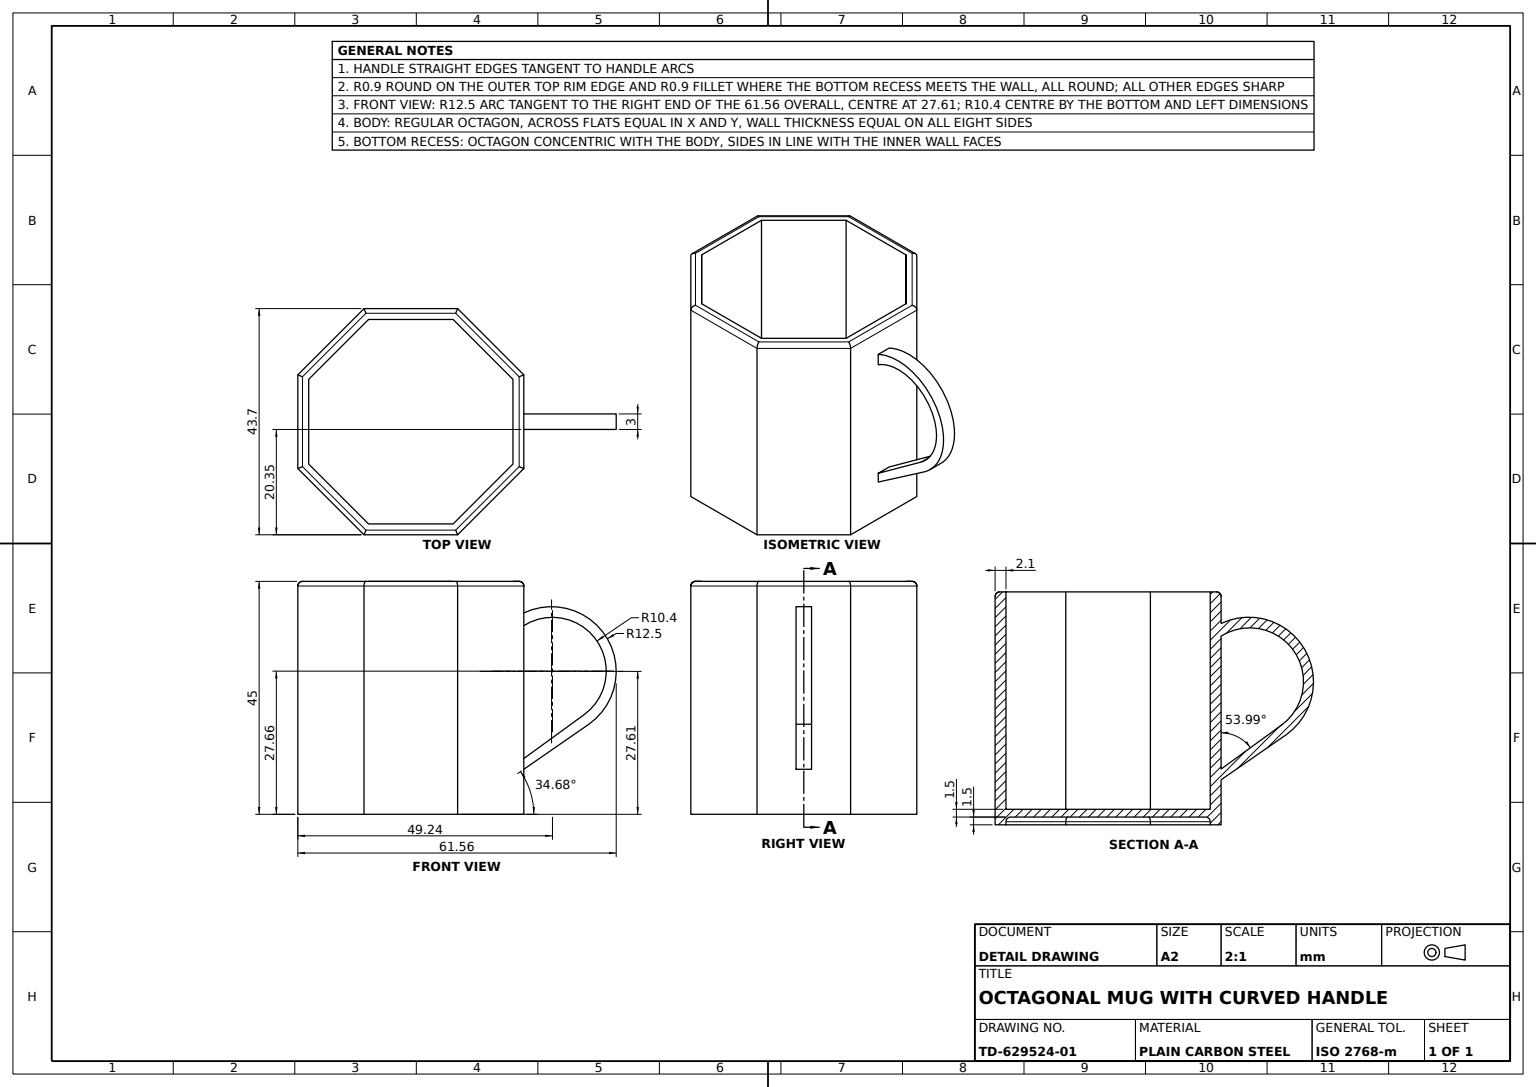
from build123d import *

# Parameters (mm, degrees)
OCTAGON_WALL_45MM_DEPTH    = 45
BOTTOM_START               = -3
BOTTOM_PLATE_1_5MM_DEPTH   = 1.5
BOTTOM_PLATE_FILLET_R0_9_R = 0.9
HANDLE_3MM_DEPTH           = 1.5
WALL_EDGE_FILLET_R0_9_R    = 0.9


with BuildPart() as part:
    # Octagon Wall Profile → Octagon Wall 45mm (new body)
    with BuildSketch(Plane(origin=(0, 0, 0), x_dir=(1, 0, 0), z_dir=(0, 1, 0))):
        Polygon((21.848632739, -9.05), (21.848632739, 9.05), (9.05, 21.848632739), (-9.05, 21.848632739), (-21.848632739, 9.05), (-21.848632739, -9.05), (-9.05, -21.848632739), (9.05, -21.848632739), align=None)
        Polygon((-19.748632739, 8.180151519), (-19.748632739, -8.180151519), (-8.180151519, -19.748632739), (8.180151519, -19.748632739), (19.748632739, -8.180151519), (19.748632739, 8.180151519), (8.180151519, 19.748632739), (-8.180151519, 19.748632739), align=None, mode=Mode.SUBTRACT)
    extrude(amount=OCTAGON_WALL_45MM_DEPTH)

    # Bottom Plate Profile → Bottom Plate 1.5mm (add)
    with BuildSketch(Plane.XZ.offset(BOTTOM_START)):
        Polygon((19.748632739, -8.180151519), (19.748632739, 8.180151519), (8.180151519, 19.748632739), (-8.180151519, 19.748632739), (-19.748632739, 8.180151519), (-19.748632739, -8.180151519), (-8.180151519, -19.748632739), (8.180151519, -19.748632739), align=None)
    extrude(amount=BOTTOM_PLATE_1_5MM_DEPTH)

    # Bottom Plate Fillet R0.9
    bottom_plate_fillet_r0_9_edges = [part.edges().sort_by_distance(p)[0] for p in [
        (13.964392129, 1.5, -13.964392129),
        (19.748632739, 1.5, 0),
        (13.964392129, 1.5, 13.964392129),
        (0, 1.5, 19.748632739),
        (-13.964392129, 1.5, 13.964392129),
        (-19.748632739, 1.5, 0),
        (-13.964392129, 1.5, -13.964392129),
        (0, 1.5, -19.748632739),
    ]]
    fillet(bottom_plate_fillet_r0_9_edges, radius=BOTTOM_PLATE_FILLET_R0_9_R)

    # Handle Profile → Handle 3mm (add, symmetric)
    with BuildSketch(Plane.XY):
        with BuildLine():
            ThreePointArc((34.430505485, 17.403482342), (38.003421513, 33.925087018), (21.848632739, 38.90022015))
            Line((21.848632739, 38.90022015), (21.848632739, 36.457189456))
            ThreePointArc((21.848632739, 36.457189456), (36.001186663, 33.487250387), (33.504255362, 19.243632352))
            Line((33.504255362, 19.243632352), (21.848632739, 10.771816388))
            Line((21.848632739, 10.771816388), (21.848632739, 8.697939383))
            Line((21.848632739, 8.697939383), (34.430505485, 17.403482342))
        make_face()
    extrude(amount=HANDLE_3MM_DEPTH, both=True)

    # Wall Edge Fillet R0.9
    wall_edge_fillet_r0_9_edges = [part.edges().sort_by_distance(p)[0] for p in [
        (15.44931637, 45, -15.44931637),
        (0, 45, -21.848632739),
        (-15.44931637, 45, -15.44931637),
        (-21.848632739, 45, 0),
        (-15.44931637, 45, 15.44931637),
        (0, 45, 21.848632739),
        (15.44931637, 45, 15.44931637),
        (21.848632739, 45, 0),
    ]]
    fillet(wall_edge_fillet_r0_9_edges, radius=WALL_EDGE_FILLET_R0_9_R)


solid = part.part
